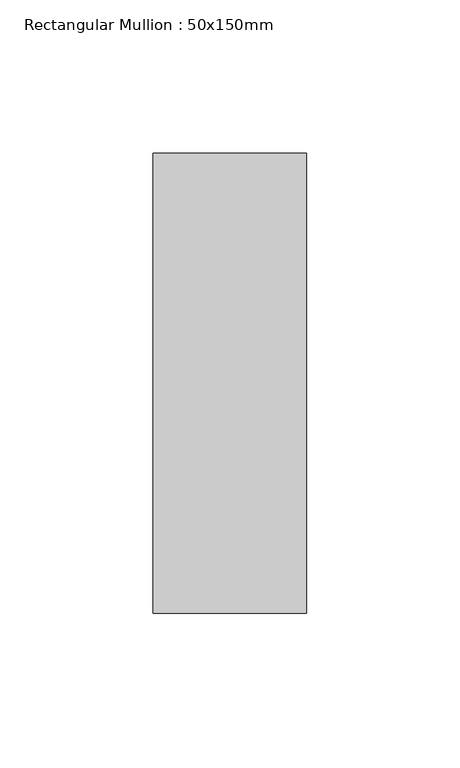
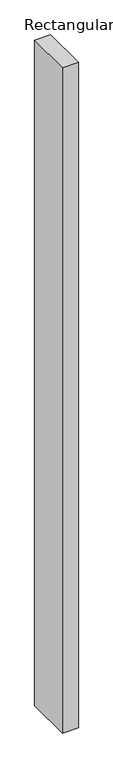
"""IFC4 building model written with IfcOpenShell, lengths in millimetres: member geometry, Rectangular Mullion : 50x150mm."""

from ifc_helpers import new_model, si_unit, frame, origin, place, context, project, spatial, polyline, outline, extrude, source, transform, mapped, element, save


def rectangular_mullion_50x150mm_7f05dd67(model_context):
    return source(origin(), model_context, "Body", "SweptSolid", [
        extrude(outline(polyline([(0.0, 75.0), (0.0, -75.0), (-50.0, -75.0), (-50.0, 75.0), (0.0, 75.0)])), frame((0.0, 0.0, -2202.7143587), z_axis=(0.0, 0.0, 1.0), x_axis=(1.0, 0.0, 0.0)), (0.0, 0.0, 1.0), 2202.7143587),
    ])


if __name__ == "__main__":
    model = new_model("IFC4")
    model_context = context("Model", 3, world=origin())
    ifc_project = project(units=[si_unit("LENGTHUNIT", "METRE", prefix="MILLI")], contexts=[model_context])
    site = spatial("IfcSite", under=ifc_project)
    building = spatial("IfcBuilding", under=site)
    placement = place(None, origin())
    rectangular_mullion_50x150mm_shape = rectangular_mullion_50x150mm_7f05dd67(model_context)
    element("IfcMember", 1, ObjectType="Rectangular Mullion : 50x150mm", at=placement, inside=building, context=model_context, shape_type="MappedRepresentation", body=[
        mapped(rectangular_mullion_50x150mm_shape, transform((0.0, 0.0, 0.0), x_axis=(1.0, 0.0, 0.0), y_axis=(0.0, 1.0, 0.0), z_axis=(0.0, 0.0, 1.0))),
    ])
    save(model, "model.ifc")

# Revit data of these elements
# Type "Rectangular Mullion : 50x150mm"
#   Keynote = "H11"
#   built-in parameter 1007304 = 0.492126 (stored number, unit not read)
#   built-in parameter 1007301 = 0.082021 (stored number, unit not read)
#   built-in parameter 1007300 = 0.082021 (stored number, unit not read)
# Element 1 (IfcMember, "Rectangular Mullion : 50x150mm")
#   Materials on its faces: "Aluminium"
# Materials
#   "Aluminium": class "Metal", colour RGB 247 247 247, transparency 0, Description = "Aluminium 6061", Cost = 0
